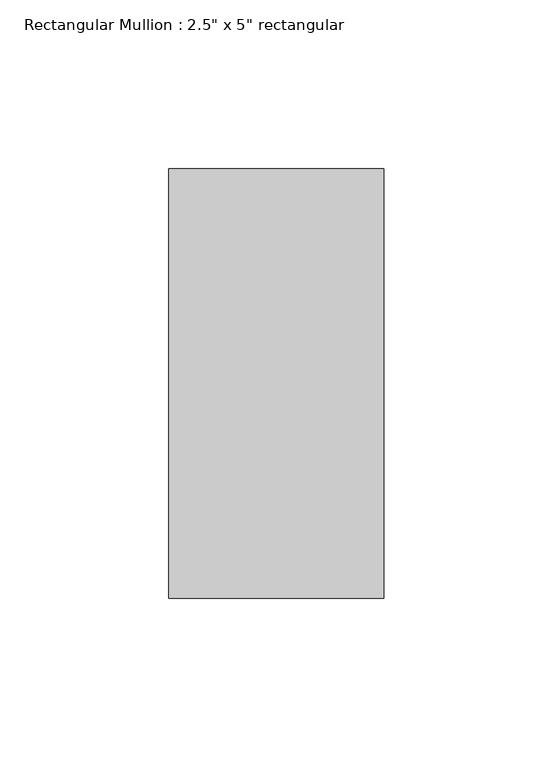
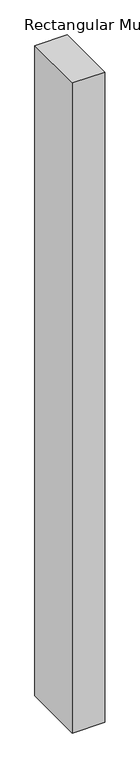
"""IFC4 building model written with IfcOpenShell, lengths in millimetres: member geometry."""

from ifc_helpers import new_model, si_unit, frame, origin, place, context, project, spatial, polyline, outline, extrude, source, transform, mapped, element, save


def member_c0163ebe(model_context):
    return source(origin(), model_context, "Body", "SweptSolid", [
        extrude(outline(polyline([(0.0, 63.5), (0.0, -63.5), (-63.5, -63.5), (-63.5, 63.5), (0.0, 63.5)])), frame((0.0, 0.0, -1348.9870163), z_axis=(0.0, 0.0, 1.0), x_axis=(1.0, 0.0, 0.0)), (0.0, 0.0, 1.0), 1348.9870163),
    ])


if __name__ == "__main__":
    model = new_model("IFC4")
    model_context = context("Model", 3, world=origin())
    ifc_project = project(units=[si_unit("LENGTHUNIT", "METRE", prefix="MILLI")], contexts=[model_context])
    site = spatial("IfcSite", under=ifc_project)
    building = spatial("IfcBuilding", under=site)
    placement = place(None, origin())
    member_shape = member_c0163ebe(model_context)
    element("IfcMember", 1, ObjectType="Rectangular Mullion : 2.5\" x 5\" rectangular", at=placement, inside=building, context=model_context, shape_type="MappedRepresentation", body=[
        mapped(member_shape, transform((0.0, 0.0, 0.0), x_axis=(1.0, 0.0, 0.0), y_axis=(0.0, 1.0, 0.0), z_axis=(0.0, 0.0, 1.0))),
    ])
    save(model, "model.ifc")

# Revit data of these elements
# Type "Rectangular Mullion : 2.5\" x 5\" rectangular"
#   built-in parameter 1007304 = 0.416667 (stored number, unit not read)
#   built-in parameter 1007301 = 0.104167 (stored number, unit not read)
#   built-in parameter 1007300 = 0.104167 (stored number, unit not read)
# Element 1 (IfcMember, "Rectangular Mullion : 2.5\" x 5\" rectangular")
#   Materials on its faces: "Aluminum"
# Materials
#   "Aluminum": class "Metal", colour RGB 247 247 247, transparency 0, Description = "Aluminum 6061", Cost = 0
